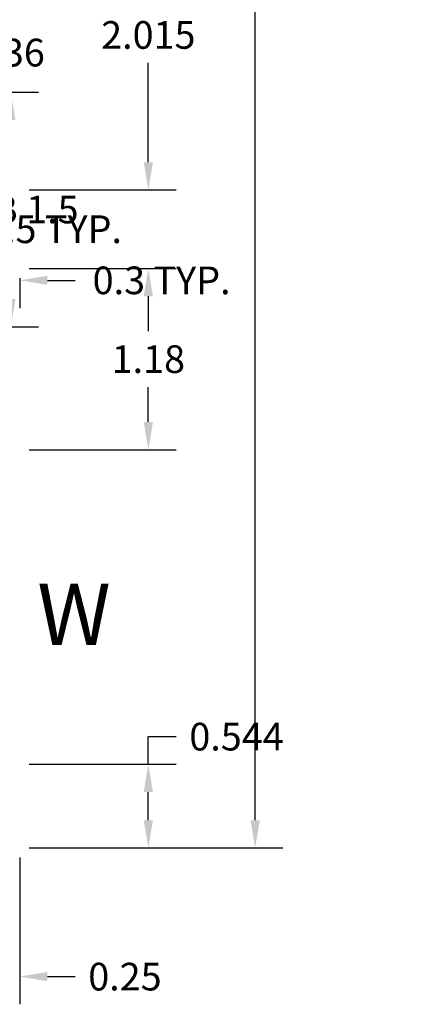
# Model space of a CAD drawing. Units: metres. Extents: x 3.9 to 21.3, y 24.8 to 56.5.
# Tile 3 of 6: x 15.8 to 18.3, y 24.8 to 31.2. Entities that reach past the tile are written whole.
import ezdxf

# ---------------------------------------------------------------- set-up
doc = ezdxf.new("R2010")
doc.units = ezdxf.units.M
doc.header["$MEASUREMENT"] = 0
doc.layers.add('DIMENSIONS', color=2, linetype='Continuous', lineweight=18)
doc.layers.add('TEXT', color=3, linetype='Continuous', lineweight=18)
doc.styles.get("Standard").update_dxf_attribs({"font": 'arial.ttf'})
doc.dimstyles.get("Standard").update_dxf_attribs({"dimtxt": 0.18, "dimasz": 0.18, "dimexe": 0.18, "dimexo": 0.0625, "dimgap": 0.09, "dimtad": 0, "dimtih": 1, "dimtoh": 1, "dimdec": 1, "dimzin": 0, "dimdsep": 46, "dimtxsty": 'Standard', "dimcen": 0.09, "dimadec": 0, "dimazin": 0, "dimtfac": 1, "dimtdec": 1, "dimtofl": 0, "dimtmove": 0, "dimatfit": 3, "dimfxl": 1, "dimtolj": 1, "dimtzin": 0, "dimarcsym": 0})

# ---------------------------------------------------------------- blocks, each defined once
blk = doc.blocks.new('*D21')
at = {"layer": 'Defpoints', "color": 0, "transparency": 16777216}
for p in [(15.7571, 38.8951), (15.7571, 25.8451), (17.2883, 25.8451)]:
    blk.add_point(p, dxfattribs=at)
at = {"layer": 'DIMENSIONS', "color": 0, "lineweight": -2, "transparency": 16777216}
for p, q in [((15.8196, 38.8951), (17.4683, 38.8951)), ((17.2883, 38.7151), (17.2883, 32.8688)), ((17.2883, 26.0251), (17.2883, 31.8713)), ((15.8196, 25.8451), (17.4683, 25.8451))]:
    blk.add_line(p, q, dxfattribs=at)
at = {"layer": 'DIMENSIONS', "color": 0, "transparency": 16777216}
for points in [[(17.2583, 38.7151), (17.3183, 38.7151), (17.2883, 38.8951)], [(17.2583, 26.0251), (17.3183, 26.0251), (17.2883, 25.8451)]]:
    blk.add_solid(points, dxfattribs=at)
at = {"layer": 'DIMENSIONS', "color": 0, "transparency": 16777216, "insert": (17.2883, 32.3701), "char_height": 0.18, "attachment_point": 5}
blk.add_mtext('\\A1;{\\H4.44444x;13.1}', dxfattribs=at)
blk = doc.blocks.new('*D47')
at = {"layer": 'Defpoints', "color": 0, "transparency": 16777216}
for p in [(15.5071, 30.1245), (15.4304, 29.6129), (15.5071, 29.6129)]:
    blk.add_point(p, dxfattribs=at)
at = {"layer": 'DIMENSIONS', "color": 0, "lineweight": -2, "transparency": 16777216}
for p, q in [((15.4304, 30.3045), (15.4304, 30.4845)), ((15.4446, 30.1245), (15.2504, 30.1245)), ((15.4446, 29.6129), (15.2504, 29.6129)), ((15.4304, 29.4329), (15.4304, 29.2529))]:
    blk.add_line(p, q, dxfattribs=at)
at = {"layer": 'DIMENSIONS', "color": 0, "transparency": 16777216}
for points in [[(15.4004, 30.3045), (15.4604, 30.3045), (15.4304, 30.1245)], [(15.4004, 29.4329), (15.4604, 29.4329), (15.4304, 29.6129)]]:
    blk.add_solid(points, dxfattribs=at)
at = {"layer": 'DIMENSIONS', "color": 0, "transparency": 16777216, "insert": (15.4304, 29.8687), "char_height": 0.18, "attachment_point": 5}
blk.add_mtext('\\A1;WINDOW 0.5 TYP.', dxfattribs=at)
blk = doc.blocks.new('*D48')
at = {"layer": 'Defpoints', "color": 0, "transparency": 16777216}
for p in [(15.5071, 29.6129), (15.7571, 29.6129), (15.7571, 29.5362)]:
    blk.add_point(p, dxfattribs=at)
at = {"layer": 'DIMENSIONS', "color": 0, "lineweight": -2, "transparency": 16777216}
for p, q in [((15.3271, 29.5362), (15.1471, 29.5362)), ((15.5071, 29.5504), (15.5071, 29.3562)), ((15.7571, 29.5504), (15.7571, 29.3562)), ((15.9371, 29.5362), (16.1171, 29.5362))]:
    blk.add_line(p, q, dxfattribs=at)
at = {"layer": 'DIMENSIONS', "color": 0, "transparency": 16777216}
for points in [[(15.3271, 29.5662), (15.3271, 29.5062), (15.5071, 29.5362)], [(15.9371, 29.5662), (15.9371, 29.5062), (15.7571, 29.5362)]]:
    blk.add_solid(points, dxfattribs=at)
at = {"layer": 'DIMENSIONS', "color": 0, "transparency": 16777216, "insert": (16.6801, 29.5362), "char_height": 0.18, "attachment_point": 5}
blk.add_mtext('\\A1;0.3 TYP.', dxfattribs=at)
blk = doc.blocks.new('*D67')
at = {"layer": 'Defpoints', "color": 0, "transparency": 16777216}
for p in [(15.4709, 30.7589), (15.6995, 30.7589), (15.4709, 29.2349)]:
    blk.add_point(p, dxfattribs=at)
at = {"layer": 'DIMENSIONS', "color": 0, "lineweight": -2, "transparency": 16777216}
for p, q in [((15.5334, 30.7589), (15.8795, 30.7589)), ((15.6995, 30.5789), (15.6995, 30.1788)), ((15.6995, 29.4149), (15.6995, 29.8149)), ((15.5334, 29.2349), (15.8795, 29.2349))]:
    blk.add_line(p, q, dxfattribs=at)
at = {"layer": 'DIMENSIONS', "color": 0, "transparency": 16777216}
for points in [[(15.6695, 30.5789), (15.7295, 30.5789), (15.6995, 30.7589)], [(15.6695, 29.4149), (15.7295, 29.4149), (15.6995, 29.2349)]]:
    blk.add_solid(points, dxfattribs=at)
at = {"layer": 'DIMENSIONS', "color": 0, "transparency": 16777216, "insert": (15.6995, 29.9969), "char_height": 0.18, "attachment_point": 5}
blk.add_mtext('\\A1;TUB 1.5', dxfattribs=at)
blk = doc.blocks.new('*D88')
at = {"layer": 'Defpoints', "color": 0, "transparency": 16777216}
for p in [(15.7571, 26.3891), (16.5936, 26.3891), (15.7571, 25.8451)]:
    blk.add_point(p, dxfattribs=at)
at = {"layer": 'DIMENSIONS', "color": 0, "lineweight": -2, "transparency": 16777216}
for p, q in [((16.5936, 26.3891), (16.5936, 26.5691)), ((16.5936, 26.5691), (16.7736, 26.5691)), ((15.8196, 26.3891), (16.7736, 26.3891)), ((16.5936, 26.0251), (16.5936, 26.2091)), ((15.8196, 25.8451), (16.7736, 25.8451))]:
    blk.add_line(p, q, dxfattribs=at)
at = {"layer": 'DIMENSIONS', "color": 0, "transparency": 16777216}
for points in [[(16.5636, 26.2091), (16.6236, 26.2091), (16.5936, 26.3891)], [(16.5636, 26.0251), (16.6236, 26.0251), (16.5936, 25.8451)]]:
    blk.add_solid(points, dxfattribs=at)
at = {"layer": 'DIMENSIONS', "color": 0, "transparency": 16777216, "insert": (17.167, 26.5691), "char_height": 0.18, "attachment_point": 5}
blk.add_mtext('\\A1;0.544', dxfattribs=at)
blk = doc.blocks.new('*D89')
at = {"layer": 'Defpoints', "color": 0, "transparency": 16777216}
for p in [(15.7571, 29.6129), (16.5936, 29.6129), (15.7571, 28.4352)]:
    blk.add_point(p, dxfattribs=at)
at = {"layer": 'DIMENSIONS', "color": 0, "lineweight": -2, "transparency": 16777216}
for p, q in [((15.8196, 29.6129), (16.7736, 29.6129)), ((16.5936, 29.4329), (16.5936, 29.206)), ((16.5936, 28.6152), (16.5936, 28.8422)), ((15.8196, 28.4352), (16.7736, 28.4352))]:
    blk.add_line(p, q, dxfattribs=at)
at = {"layer": 'DIMENSIONS', "color": 0, "transparency": 16777216}
for points in [[(16.5636, 29.4329), (16.6236, 29.4329), (16.5936, 29.6129)], [(16.5636, 28.6152), (16.6236, 28.6152), (16.5936, 28.4352)]]:
    blk.add_solid(points, dxfattribs=at)
at = {"layer": 'DIMENSIONS', "color": 0, "transparency": 16777216, "insert": (16.5936, 29.0241), "char_height": 0.18, "attachment_point": 5}
blk.add_mtext('\\A1;1.18', dxfattribs=at)
blk = doc.blocks.new('*D90')
at = {"layer": 'Defpoints', "color": 0, "transparency": 16777216}
for p in [(15.7571, 32.1396), (16.5936, 32.1396), (15.7571, 30.1245)]:
    blk.add_point(p, dxfattribs=at)
at = {"layer": 'DIMENSIONS', "color": 0, "lineweight": -2, "transparency": 16777216}
for p, q in [((15.8196, 32.1396), (16.7736, 32.1396)), ((16.5936, 31.9596), (16.5936, 31.3139)), ((16.5936, 30.3045), (16.5936, 30.9501)), ((15.8196, 30.1245), (16.7736, 30.1245))]:
    blk.add_line(p, q, dxfattribs=at)
at = {"layer": 'DIMENSIONS', "color": 0, "transparency": 16777216}
for points in [[(16.5636, 31.9596), (16.6236, 31.9596), (16.5936, 32.1396)], [(16.5636, 30.3045), (16.6236, 30.3045), (16.5936, 30.1245)]]:
    blk.add_solid(points, dxfattribs=at)
at = {"layer": 'DIMENSIONS', "color": 0, "transparency": 16777216, "insert": (16.5936, 31.132), "char_height": 0.18, "attachment_point": 5}
blk.add_mtext('\\A1;2.015', dxfattribs=at)
blk = doc.blocks.new('*D94')
at = {"layer": 'Defpoints', "color": 0, "transparency": 16777216}
for p in [(15.5071, 25.9951), (15.7571, 25.8451), (15.7571, 25.0086)]:
    blk.add_point(p, dxfattribs=at)
at = {"layer": 'DIMENSIONS', "color": 0, "lineweight": -2, "transparency": 16777216}
for p, q in [((15.5071, 25.9326), (15.5071, 24.8286)), ((15.7571, 25.7826), (15.7571, 24.8286)), ((15.3271, 25.0086), (15.1471, 25.0086)), ((15.9371, 25.0086), (16.1171, 25.0086))]:
    blk.add_line(p, q, dxfattribs=at)
at = {"layer": 'DIMENSIONS', "color": 0, "transparency": 16777216}
for points in [[(15.3271, 25.0386), (15.3271, 24.9786), (15.5071, 25.0086)], [(15.9371, 25.0386), (15.9371, 24.9786), (15.7571, 25.0086)]]:
    blk.add_solid(points, dxfattribs=at)
at = {"layer": 'DIMENSIONS', "color": 0, "transparency": 16777216, "insert": (16.4416, 25.0086), "char_height": 0.18, "attachment_point": 5}
blk.add_mtext('\\A1;0.25', dxfattribs=at)
blk = doc.blocks.new('*D112')
at = {"layer": 'Defpoints', "color": 0, "transparency": 16777216}
for p in [(15.014, 30.6573), (15.0137, 30.3017)]:
    blk.add_point(p, dxfattribs=at)
at = {"layer": 'DIMENSIONS', "color": 0, "lineweight": -2, "transparency": 16777216}
for p, q in [((15.0143, 31.0173), (15.0141, 30.8373)), ((15.1943, 31.0173), (15.0143, 31.0173)), ((15.0137, 30.2117), (15.0137, 30.3917)), ((14.9237, 30.3017), (15.1037, 30.3017))]:
    blk.add_line(p, q, dxfattribs=at)
at = {"layer": 'DIMENSIONS', "color": 0, "transparency": 16777216}
blk.add_solid([(14.9841, 30.8373), (15.0441, 30.8372), (15.014, 30.6573)], dxfattribs=at)
at = {"layer": 'DIMENSIONS', "color": 0, "transparency": 16777216, "insert": (15.6041, 31.0173), "char_height": 0.18, "attachment_point": 5}
blk.add_mtext('\\A1;R0.36', dxfattribs=at)

msp = doc.modelspace()

# ---------------------------------------------------------------- texts
at = {"layer": 'TEXT', "insert": (15.8708, 27.5649), "char_height": 0.4, "attachment_point": 1}
msp.add_mtext_dynamic_manual_height_columns('W', width=0.69425, gutter_width=1, heights=[0], dxfattribs=at)

# ---------------------------------------------------------------- dimensions: what is measured, and where the dimension line sits
at = {"layer": 'DIMENSIONS'}
for base, p1, p2, angle, text, override, picture, middle in [((17.2883128981, 25.8450722391), (15.7571276207, 38.8950722391), (15.7571276207, 25.8450722391), 90, '{\\H4.44444x;<>}', {"dimclrd": 0, "dimclre": 0, "dimclrt": 0}, '*D21', (17.2883128981, 32.3700722391)), ((15.6995, 30.7589), (15.4709, 29.2349), (15.4709, 30.7589), 90, 'TUB <>', {"dimdec": 1, "dimlfac": 1, "dimrnd": 0, "dimzin": 0, "dimdsep": 46, "dimlunit": 2}, '*D67', (15.6995, 29.9969)), ((15.4304, 29.6129), (15.5071, 30.1245), (15.5071, 29.6129), 270, 'WINDOW <> TYP.', {"dimdec": 1, "dimlfac": 1, "dimrnd": 0, "dimzin": 0, "dimdsep": 46, "dimlunit": 2}, '*D47', (15.4304, 29.8687)), ((15.7571276207, 29.536179007), (15.5071276207, 29.6129107404), (15.7571276207, 29.6129107404), 0, '<> TYP.', {"dimdec": 1, "dimlfac": 1, "dimrnd": 0, "dimzin": 0, "dimdsep": 46, "dimlunit": 2}, '*D48', (16.6801494488, 29.536179007))]:
    dim = msp.add_linear_dim(base=base, p1=p1, p2=p2, angle=angle, text=text, dimstyle='Standard', override=override, dxfattribs=at)
    dim.commit()
    dim.dimension.update_dxf_attribs({"geometry": picture, "text_midpoint": middle})
for base, p1, p2, override, picture, middle in [((16.5936, 32.1396), (15.7571, 30.1245), (15.7571, 32.1396), {"dimdec": 3, "dimlfac": 1, "dimrnd": 0, "dimzin": 0, "dimdsep": 46, "dimlunit": 2}, '*D90', (16.5936, 31.132)), ((16.5936, 29.6129), (15.7571, 28.4352), (15.7571, 29.6129), {"dimdec": 2, "dimlfac": 1, "dimrnd": 0, "dimzin": 0, "dimdsep": 46, "dimlunit": 2}, '*D89', (16.5936, 29.0241)), ((16.5936, 26.3891), (15.7571, 25.8451), (15.7571, 26.3891), {"dimdec": 3, "dimlfac": 1, "dimrnd": 0, "dimzin": 0, "dimdsep": 46, "dimlunit": 2}, '*D88', (17.167, 26.5691))]:
    dim = msp.add_linear_dim(base=base, p1=p1, p2=p2, angle=90, dimstyle='Standard', override=override, dxfattribs=at)
    dim.commit()
    dim.dimension.update_dxf_attribs({"geometry": picture, "text_midpoint": middle})
dim = msp.add_radius_dim(center=(15.0137, 30.3017), mpoint=(15.014, 30.6573), dimstyle='Standard', override={"dimdec": 2, "dimlfac": 1, "dimrnd": 0, "dimzin": 0, "dimdsep": 46, "dimlunit": 2}, dxfattribs=at)
dim.commit()
dim.dimension.update_dxf_attribs({"geometry": '*D112', "text_midpoint": (15.6041, 31.0173)})
dim = msp.add_linear_dim(base=(15.7571, 25.0086), p1=(15.5071, 25.9951), p2=(15.7571, 25.8451), dimstyle='Standard', override={"dimdec": 2, "dimlfac": 1, "dimrnd": 0, "dimzin": 0, "dimdsep": 46, "dimlunit": 2}, dxfattribs=at)
dim.commit()
dim.dimension.update_dxf_attribs({"geometry": '*D94', "text_midpoint": (16.4416, 25.0086)})

doc.saveas('drawing.dxf')
